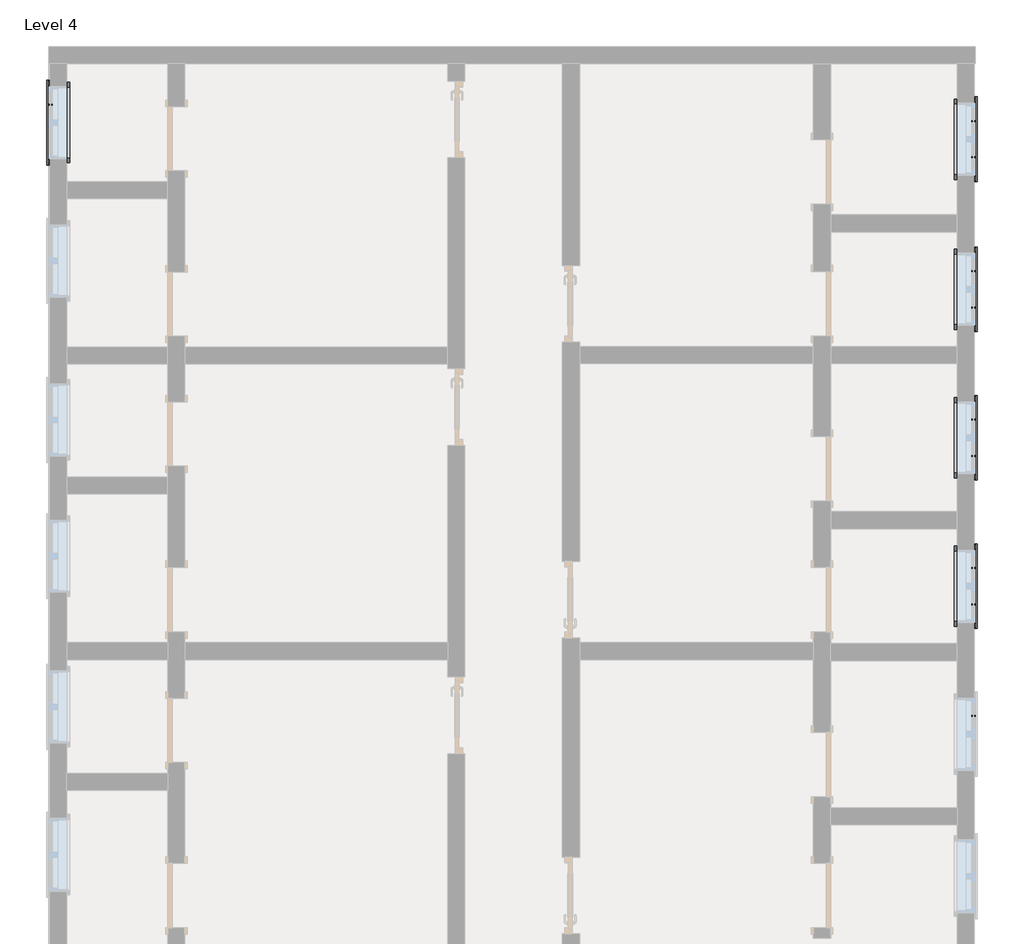
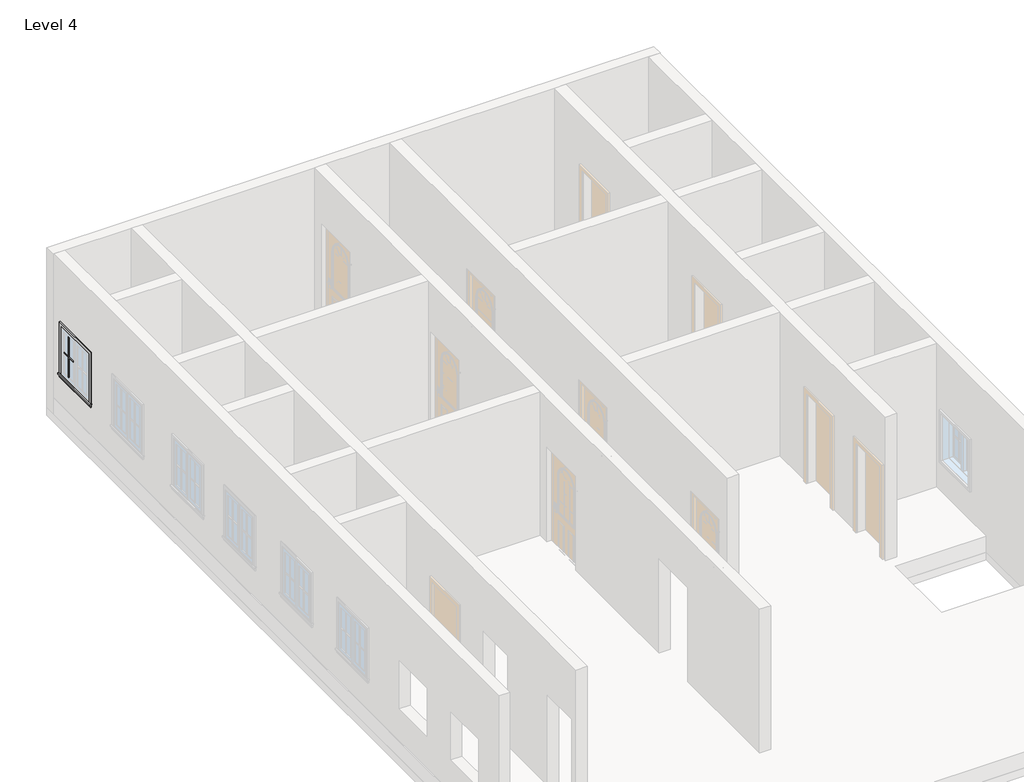
# One storey, part 4 of 4: 20 proxies.
"""IFC4 building model written with IfcOpenShell, lengths in millimetres."""

from ifc_helpers import new_model, si_unit, origin, place, context, project, spatial, transform, mapped, element, save
from components import muntin_pattern_2x2_muntin_pattern_2x2_b3fe6957, muntin_pattern_2x2_muntin_pattern_2x2_3e0ecaf2, trim_window_exterior_flat_with_sill_41619996, trim_window_interior_flat_picture_frame_51c85655

model = new_model("IFC4")

# Units and contexts
model_context = context("Model", 3, world=origin())
ifc_project = project(units=[si_unit("LENGTHUNIT", "METRE", prefix="MILLI")], contexts=[model_context])

# Site, building, storey
site = spatial("IfcSite", under=ifc_project)
building = spatial("IfcBuilding", under=site)
storey = spatial("IfcBuildingStorey", under=building, Name="Level 4", Elevation=9144.0)

# Proxies
placement = place(None, origin())
muntin_pattern_2x2_muntin_pattern_2x2_shape = muntin_pattern_2x2_muntin_pattern_2x2_b3fe6957(model_context)
element("IfcBuildingElementProxy", 1, Name="Muntin Pattern_2x2 : Muntin Pattern_2x2", ObjectType="Muntin Pattern_2x2 : Muntin Pattern_2x2", at=placement, inside=storey, context=model_context, shape_type="MappedRepresentation", body=[
    mapped(muntin_pattern_2x2_muntin_pattern_2x2_shape, transform((4489.4641134, 66.1024728, 10128.25), x_axis=(0.0, -1.0, 0.0), y_axis=(1.0, 0.0, 0.0), z_axis=(0.0, 0.0, 1.0))),
])
element("IfcBuildingElementProxy", 2, Name="Muntin Pattern_2x2 : Muntin Pattern_2x2", ObjectType="Muntin Pattern_2x2 : Muntin Pattern_2x2", at=placement, inside=storey, context=model_context, shape_type="MappedRepresentation", body=[
    mapped(muntin_pattern_2x2_muntin_pattern_2x2_shape, transform((4489.4641134, 1818.7024728, 10128.25), x_axis=(0.0, -1.0, 0.0), y_axis=(1.0, 0.0, 0.0), z_axis=(0.0, 0.0, 1.0))),
])
element("IfcBuildingElementProxy", 3, Name="Muntin Pattern_2x2 : Muntin Pattern_2x2", ObjectType="Muntin Pattern_2x2 : Muntin Pattern_2x2", at=placement, inside=storey, context=model_context, shape_type="MappedRepresentation", body=[
    mapped(muntin_pattern_2x2_muntin_pattern_2x2_shape, transform((4489.4641134, 3577.6524728, 10128.25), x_axis=(0.0, -1.0, 0.0), y_axis=(1.0, 0.0, 0.0), z_axis=(0.0, 0.0, 1.0))),
])
element("IfcBuildingElementProxy", 4, Name="Muntin Pattern_2x2 : Muntin Pattern_2x2", ObjectType="Muntin Pattern_2x2 : Muntin Pattern_2x2", at=placement, inside=storey, context=model_context, shape_type="MappedRepresentation", body=[
    mapped(muntin_pattern_2x2_muntin_pattern_2x2_shape, transform((4489.4641134, 5336.6024728, 10128.25), x_axis=(0.0, -1.0, 0.0), y_axis=(1.0, 0.0, 0.0), z_axis=(0.0, 0.0, 1.0))),
])
element("IfcBuildingElementProxy", 5, Name="Muntin Pattern_2x2 : Muntin Pattern_2x2", ObjectType="Muntin Pattern_2x2 : Muntin Pattern_2x2", at=placement, inside=storey, context=model_context, shape_type="MappedRepresentation", body=[
    mapped(muntin_pattern_2x2_muntin_pattern_2x2_shape, transform((4489.4641134, 7114.6024728, 10128.25), x_axis=(0.0, -1.0, 0.0), y_axis=(1.0, 0.0, 0.0), z_axis=(0.0, 0.0, 1.0))),
])
muntin_pattern_2x2_muntin_pattern_2x2_2_shape = muntin_pattern_2x2_muntin_pattern_2x2_3e0ecaf2(model_context)
element("IfcBuildingElementProxy", 6, Name="Muntin Pattern_2x2 : Muntin Pattern_2x2", ObjectType="Muntin Pattern_2x2 : Muntin Pattern_2x2", at=placement, inside=storey, context=model_context, shape_type="MappedRepresentation", body=[
    mapped(muntin_pattern_2x2_muntin_pattern_2x2_2_shape, transform((-6438.8858866, 7311.4524728, 10128.25), x_axis=(0.0, -1.0, 0.0), y_axis=(1.0, 0.0, 0.0), z_axis=(0.0, 0.0, 1.0))),
])
element("IfcBuildingElementProxy", 7, Name="Muntin Pattern_2x2 : Muntin Pattern_2x2", ObjectType="Muntin Pattern_2x2 : Muntin Pattern_2x2", at=placement, inside=storey, context=model_context, shape_type="MappedRepresentation", body=[
    mapped(muntin_pattern_2x2_muntin_pattern_2x2_2_shape, transform((4489.4641134, 1390.0774728, 10128.25), x_axis=(0.0, 1.0, 0.0), y_axis=(-1.0, 0.0, 0.0), z_axis=(0.0, 0.0, 1.0))),
])
element("IfcBuildingElementProxy", 8, Name="Muntin Pattern_2x2 : Muntin Pattern_2x2", ObjectType="Muntin Pattern_2x2 : Muntin Pattern_2x2", at=placement, inside=storey, context=model_context, shape_type="MappedRepresentation", body=[
    mapped(muntin_pattern_2x2_muntin_pattern_2x2_2_shape, transform((4489.4641134, 3149.0274728, 10128.25), x_axis=(0.0, 1.0, 0.0), y_axis=(-1.0, 0.0, 0.0), z_axis=(0.0, 0.0, 1.0))),
])
element("IfcBuildingElementProxy", 9, Name="Muntin Pattern_2x2 : Muntin Pattern_2x2", ObjectType="Muntin Pattern_2x2 : Muntin Pattern_2x2", at=placement, inside=storey, context=model_context, shape_type="MappedRepresentation", body=[
    mapped(muntin_pattern_2x2_muntin_pattern_2x2_2_shape, transform((4489.4641134, 4907.9774728, 10128.25), x_axis=(0.0, 1.0, 0.0), y_axis=(-1.0, 0.0, 0.0), z_axis=(0.0, 0.0, 1.0))),
])
element("IfcBuildingElementProxy", 10, Name="Muntin Pattern_2x2 : Muntin Pattern_2x2", ObjectType="Muntin Pattern_2x2 : Muntin Pattern_2x2", at=placement, inside=storey, context=model_context, shape_type="MappedRepresentation", body=[
    mapped(muntin_pattern_2x2_muntin_pattern_2x2_2_shape, transform((4489.4641134, 6685.9774728, 10128.25), x_axis=(0.0, 1.0, 0.0), y_axis=(-1.0, 0.0, 0.0), z_axis=(0.0, 0.0, 1.0))),
])
trim_window_exterior_flat_with_sill_shape = trim_window_exterior_flat_with_sill_41619996(model_context)
element("IfcBuildingElementProxy", 11, Name="Trim-Window-Exterior-Flat : with Sill", ObjectType="Trim-Window-Exterior-Flat : with Sill", at=placement, inside=storey, context=model_context, shape_type="MappedRepresentation", body=[
    mapped(trim_window_exterior_flat_with_sill_shape, transform((-6448.4108866, 7097.1399728, 10972.8), x_axis=(0.0, -1.0, 0.0), y_axis=(0.0, 0.0, 1.0), z_axis=(-1.0, 0.0, 0.0))),
])
element("IfcBuildingElementProxy", 12, Name="Trim-Window-Exterior-Flat : with Sill", ObjectType="Trim-Window-Exterior-Flat : with Sill", at=placement, inside=storey, context=model_context, shape_type="MappedRepresentation", body=[
    mapped(trim_window_exterior_flat_with_sill_shape, transform((4498.9891134, 1604.3899728, 10972.8), x_axis=(0.0, 1.0, 0.0), y_axis=(0.0, 0.0, 1.0), z_axis=(1.0, 0.0, 0.0))),
])
element("IfcBuildingElementProxy", 13, Name="Trim-Window-Exterior-Flat : with Sill", ObjectType="Trim-Window-Exterior-Flat : with Sill", at=placement, inside=storey, context=model_context, shape_type="MappedRepresentation", body=[
    mapped(trim_window_exterior_flat_with_sill_shape, transform((4498.9891134, 3363.3399728, 10972.8), x_axis=(0.0, 1.0, 0.0), y_axis=(0.0, 0.0, 1.0), z_axis=(1.0, 0.0, 0.0))),
])
element("IfcBuildingElementProxy", 14, Name="Trim-Window-Exterior-Flat : with Sill", ObjectType="Trim-Window-Exterior-Flat : with Sill", at=placement, inside=storey, context=model_context, shape_type="MappedRepresentation", body=[
    mapped(trim_window_exterior_flat_with_sill_shape, transform((4498.9891134, 5122.2899728, 10972.8), x_axis=(0.0, 1.0, 0.0), y_axis=(0.0, 0.0, 1.0), z_axis=(1.0, 0.0, 0.0))),
])
element("IfcBuildingElementProxy", 15, Name="Trim-Window-Exterior-Flat : with Sill", ObjectType="Trim-Window-Exterior-Flat : with Sill", at=placement, inside=storey, context=model_context, shape_type="MappedRepresentation", body=[
    mapped(trim_window_exterior_flat_with_sill_shape, transform((4498.9891134, 6900.2899728, 10972.8), x_axis=(0.0, 1.0, 0.0), y_axis=(0.0, 0.0, 1.0), z_axis=(1.0, 0.0, 0.0))),
])
trim_window_interior_flat_picture_frame_shape = trim_window_interior_flat_picture_frame_51c85655(model_context)
element("IfcBuildingElementProxy", 16, Name="Trim-Window-Interior-Flat : Picture Frame", ObjectType="Trim-Window-Interior-Flat : Picture Frame", at=placement, inside=storey, context=model_context, shape_type="MappedRepresentation", body=[
    mapped(trim_window_interior_flat_picture_frame_shape, transform((-6245.2108866, 7097.1399728, 10972.8), x_axis=(0.0, 1.0, 0.0), y_axis=(0.0, 0.0, 1.0), z_axis=(1.0, 0.0, 0.0))),
])
element("IfcBuildingElementProxy", 17, Name="Trim-Window-Interior-Flat : Picture Frame", ObjectType="Trim-Window-Interior-Flat : Picture Frame", at=placement, inside=storey, context=model_context, shape_type="MappedRepresentation", body=[
    mapped(trim_window_interior_flat_picture_frame_shape, transform((4295.7891134, 1604.3899728, 10972.8), x_axis=(0.0, -1.0, 0.0), y_axis=(0.0, 0.0, 1.0), z_axis=(-1.0, 0.0, 0.0))),
])
element("IfcBuildingElementProxy", 18, Name="Trim-Window-Interior-Flat : Picture Frame", ObjectType="Trim-Window-Interior-Flat : Picture Frame", at=placement, inside=storey, context=model_context, shape_type="MappedRepresentation", body=[
    mapped(trim_window_interior_flat_picture_frame_shape, transform((4295.7891134, 3363.3399728, 10972.8), x_axis=(0.0, -1.0, 0.0), y_axis=(0.0, 0.0, 1.0), z_axis=(-1.0, 0.0, 0.0))),
])
element("IfcBuildingElementProxy", 19, Name="Trim-Window-Interior-Flat : Picture Frame", ObjectType="Trim-Window-Interior-Flat : Picture Frame", at=placement, inside=storey, context=model_context, shape_type="MappedRepresentation", body=[
    mapped(trim_window_interior_flat_picture_frame_shape, transform((4295.7891134, 5122.2899728, 10972.8), x_axis=(0.0, -1.0, 0.0), y_axis=(0.0, 0.0, 1.0), z_axis=(-1.0, 0.0, 0.0))),
])
element("IfcBuildingElementProxy", 20, Name="Trim-Window-Interior-Flat : Picture Frame", ObjectType="Trim-Window-Interior-Flat : Picture Frame", at=placement, inside=storey, context=model_context, shape_type="MappedRepresentation", body=[
    mapped(trim_window_interior_flat_picture_frame_shape, transform((4295.7891134, 6900.2899728, 10972.8), x_axis=(0.0, -1.0, 0.0), y_axis=(0.0, 0.0, 1.0), z_axis=(-1.0, 0.0, 0.0))),
])

save(model, "model.ifc")

# Revit data of these elements
# Type "Muntin Pattern_2x2 : Muntin Pattern_2x2"
#   Width [instance default] = 4' - 0"
#   Thickness = 0' - 0 1/2"
#   Height [instance default] = 4' - 0"
#   Distance = 0' - 0 3/4"
#   Interior Material [instance default] = none
#   Exterior Material [instance default] = none
#   Default Elevation = 0
# Type "Trim-Window-Exterior-Flat : with Sill"
#   Trim Width = 0' - 2 1/4"
#   Trim Thickness_Picture Frame = 0' - 1 1/4"
#   Trim Thickness_with Sill = 0' - 0 3/4"
#   Sill Thickness = 0' - 1 1/4"
#   Opening Width [instance default] = 2' - 0"
#   Opening Height [instance default] = 3' - 0"
#   Default Elevation = 4' - 0"
#   Sill = yes
#   Picture Frame = no
#   Trim Material [instance default] = none
# Type "Trim-Window-Interior-Flat : Picture Frame"
#   Trim Thickness_Picture Frame = 0' - 1 1/4"
#   Trim Width = 0' - 2 1/4"
#   Trim Thickness_with Sill = 0' - 0 3/4"
#   Sill Thickness = 0' - 1 1/4"
#   Opening Width [instance default] = 2' - 0"
#   Opening Height [instance default] = 3' - 0"
#   Default Elevation = 4' - 0"
#   Sill = no
#   Picture Frame = yes
#   Trim Material [instance default] = none
# Elements 1, 2, 3, 4, 5, 6, 7, 8, 9, 10 (IfcBuildingElementProxy, "Muntin Pattern_2x2 : Muntin Pattern_2x2")
#   Width = 0' - 11 5/8"
#   Height = 2' - 6 1/2"
#   Interior Material = Wood - Stained
#   Exterior Material = Clad - White
#   Phase Created = New Construction
#   Materials on its faces: "Clad - White", "Wood - Stained"
# Elements 11, 12, 13, 14, 15 (IfcBuildingElementProxy, "Trim-Window-Exterior-Flat : with Sill")
#   Opening Width = 2' - 10"
#   Opening Height = 3' - 0"
#   Trim Material = Clad - White
#   Phase Created = New Construction
#   Materials on its faces: "Clad - White"
# Elements 16, 17, 18, 19, 20 (IfcBuildingElementProxy, "Trim-Window-Interior-Flat : Picture Frame")
#   Opening Width = 2' - 10"
#   Opening Height = 3' - 0"
#   Trim Material = Wood - Stained
#   Phase Created = New Construction
#   Materials on its faces: "Wood - Stained"
# Materials
#   "Clad - White": class "Wood", colour RGB 242 242 238, transparency 0, Cost = 0
#   "Wood - Stained": class "Wood", colour RGB 224 178 126, transparency 0, Cost = 0
